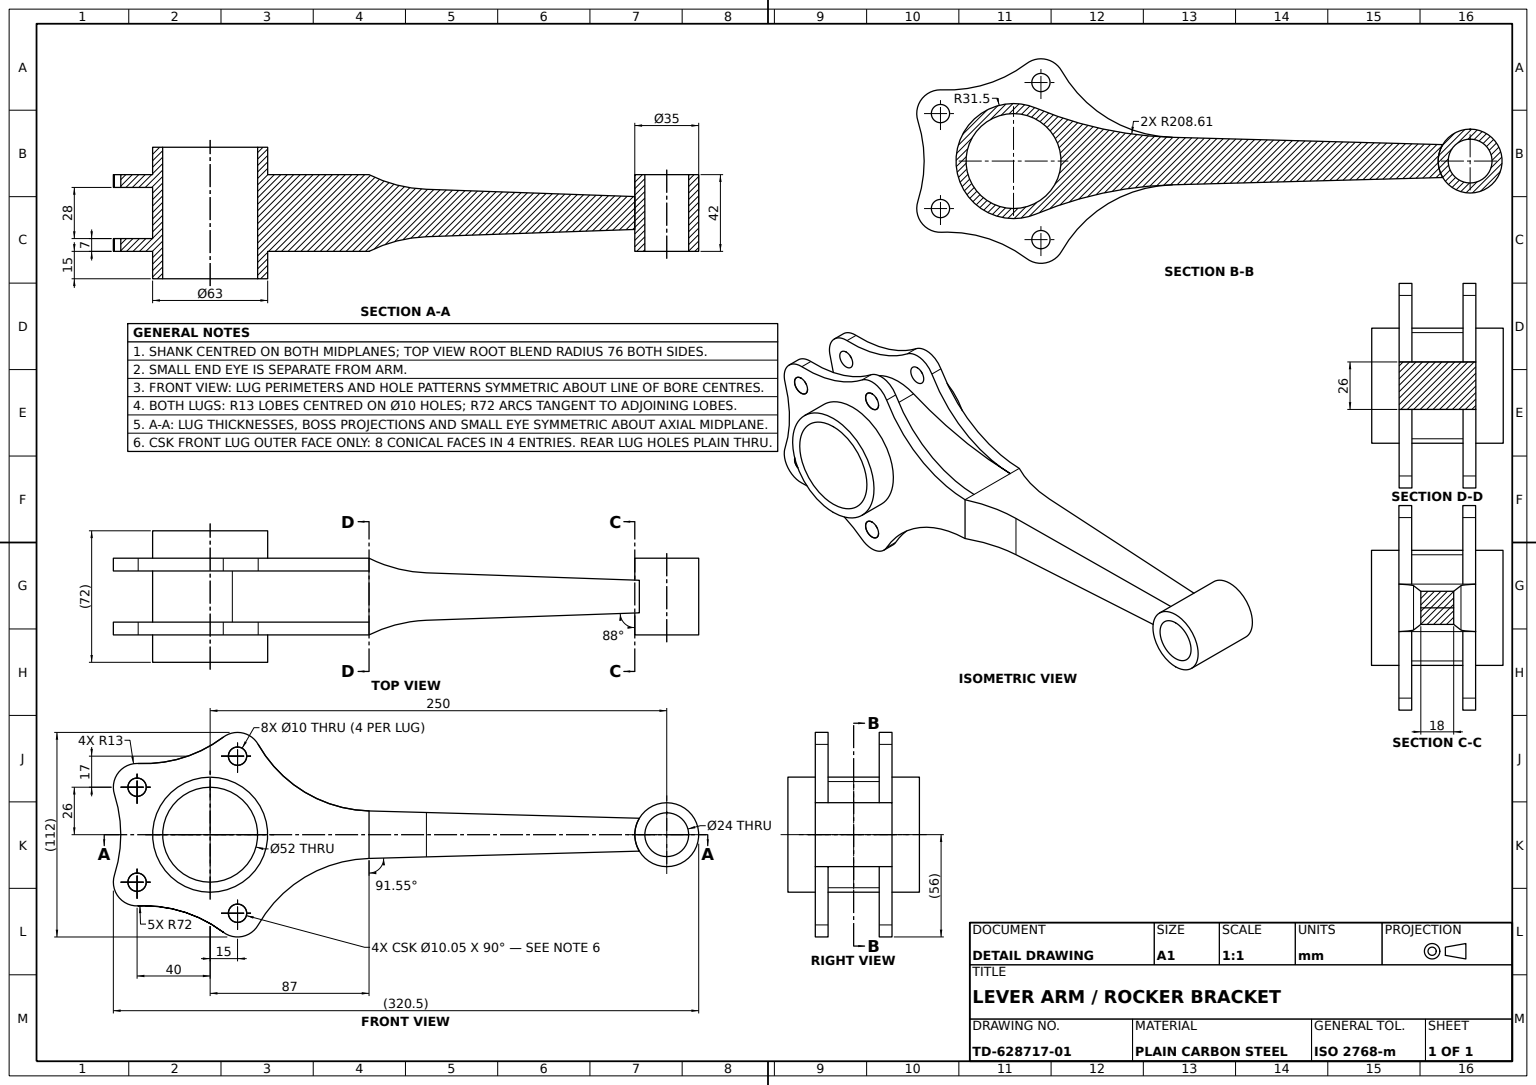
from build123d import *

# Parameters (mm, degrees)
ROD_PROFILE_SKETCH_R       = 31.5
ROD_PROFILE_SKETCH_R_2     = 26
ROD_BODY_DEPTH             = 36
SKETCH2_7_R                = 31.5
BIG_END_BOSS_DEPTH         = 21
SKETCH2_8_R                = 17.5
SKETCH2_8_R_2              = 12
SMALL_END_BOSS_DEPTH       = 21
BIG_END_CUT_DEPTH          = 14
BOLT_HOLES_10_AT_2_COUNT   = 2
BOLT_HOLES_10_AT_2_PITCH   = 57.567351858
BOLT_HOLES_10_AT_3_COUNT   = 2
BOLT_HOLES_10_AT_3_PITCH   = 86
BOLT_HOLES_10_AT_4_COUNT   = 2
BOLT_HOLES_10_AT_4_PITCH   = 88.238313674
SHANK_TAPER_CUT_DEPTH      = 276.659663353
SHANK_TAPER_CUT_DEPTH_BACK = 276.659663353


with BuildPart() as part:
    # Rod Profile Sketch → Rod Body (new, symmetric)
    with BuildSketch(Plane(origin=(0, 0, 0), x_dir=(1, 0, 0), z_dir=(0, 1, 0))):
        with Locations(Location((0, 0, 0), (0, 0, 270))):
            Circle(ROD_PROFILE_SKETCH_R)
        with Locations(Location((0, 0, 0), (0, 0, 270))):
            Circle(ROD_PROFILE_SKETCH_R_2, mode=Mode.SUBTRACT)
    extrude(amount=ROD_BODY_DEPTH, both=True)

    # Sketch2_7 → Big End Boss (add, symmetric)
    with BuildSketch(Plane(origin=(0, 0, 0), x_dir=(1, 0, 0), z_dir=(0, 1, 0))):
        with BuildLine():
            Line((86.968573361, -13), (234.99166898, -9))
            ThreePointArc((234.99166898, -9), (232.5, 0), (234.99166898, 9))
            Line((234.99166898, 9), (86.968573361, 13))
            ThreePointArc((86.968573361, 13), (51.854086448, 23.24367301), (26.304418517, 49.419511039))
            ThreePointArc((26.304418517, 49.419511039), (17.6406075, 55.72899022), (7.181946677, 53.386435492))
            ThreePointArc((7.181946677, 53.386435492), (-14.855989459, 42.122318837), (-39.406288617, 38.986435492))
            ThreePointArc((-39.406288617, 38.986435492), (-50.326951915, 33.896458963), (-52.376901133, 22.023529412))
            ThreePointArc((-52.376901133, 22.023529412), (-48.925892025, 0), (-52.376901133, -22.023529412))
            ThreePointArc((-52.376901133, -22.023529412), (-50.326951915, -33.896458963), (-39.406288617, -38.986435492))
            ThreePointArc((-39.406288617, -38.986435492), (-14.855989459, -42.122318837), (7.181946677, -53.386435492))
            ThreePointArc((7.181946677, -53.386435492), (17.6406075, -55.72899022), (26.304418517, -49.419511039))
            ThreePointArc((26.304418517, -49.419511039), (51.854086448, -23.24367301), (86.968573361, -13))
        make_face()
        with Locations(Location((0, 0, 0), (0, 0, 270))):
            Circle(SKETCH2_7_R, mode=Mode.SUBTRACT)
    extrude(amount=BIG_END_BOSS_DEPTH, both=True)

    # Big End Cut Sketch → Big End Cut (cut, symmetric)
    with BuildSketch(Plane(origin=(0, 0, 0), x_dir=(1, 0, 0), z_dir=(0, 1, 0))):
        with BuildLine():
            ThreePointArc((26.304418517, -49.419511039), (51.854086448, -23.24367301), (86.968573361, -13))
            ThreePointArc((86.968573361, -13), (48.815835223, -17.5713072), (12.14882026, -29.062968986))
            ThreePointArc((12.14882026, -29.062968986), (-31.5, 0), (12.14882026, 29.062968986))
            ThreePointArc((12.14882026, 29.062968986), (48.815835223, 17.5713072), (86.968573361, 13))
            ThreePointArc((86.968573361, 13), (51.854086448, 23.24367301), (26.304418517, 49.419511039))
            ThreePointArc((26.304418517, 49.419511039), (17.6406075, 55.72899022), (7.181946677, 53.386435492))
            ThreePointArc((7.181946677, 53.386435492), (-14.855989459, 42.122318837), (-39.406288617, 38.986435492))
            ThreePointArc((-39.406288617, 38.986435492), (-50.326951915, 33.896458963), (-52.376901133, 22.023529412))
            ThreePointArc((-52.376901133, 22.023529412), (-48.925892025, 0), (-52.376901133, -22.023529412))
            ThreePointArc((-52.376901133, -22.023529412), (-50.326951915, -33.896458963), (-39.406288617, -38.986435492))
            ThreePointArc((-39.406288617, -38.986435492), (-14.855989459, -42.122318837), (7.181946677, -53.386435492))
            ThreePointArc((7.181946677, -53.386435492), (17.6406075, -55.72899022), (26.304418517, -49.419511039))
        make_face()
    extrude(amount=BIG_END_CUT_DEPTH, both=True, mode=Mode.SUBTRACT)

    # Sketch9 → Bolt Holes _10 (revolve, cut)
    with BuildSketch(Plane(origin=(15, 21, -43), x_dir=(0, 0, 1), z_dir=(1, 0, 0))):
        Polygon((0, 0), (0, 57), (5, 57), (5, 0.025), (5.025, 0), align=None)
    bolt_holes_10 = revolve(axis=Axis((15, 27.35, -43), (0, -1, 0)), mode=Mode.SUBTRACT)

    # Bolt Holes _10 at 2: Bolt Holes _10 ×2
    with Locations(*[Vector(-0.9554026409829016, 0, 0.29530627084926053) * (i * BOLT_HOLES_10_AT_2_PITCH) for i in range(1, BOLT_HOLES_10_AT_2_COUNT)]):
        add(bolt_holes_10, mode=Mode.SUBTRACT)

    # Bolt Holes _10 at 3: Bolt Holes _10 ×2
    with Locations(*[(0, 0, i * BOLT_HOLES_10_AT_3_PITCH) for i in range(1, BOLT_HOLES_10_AT_3_COUNT)]):
        add(bolt_holes_10, mode=Mode.SUBTRACT)

    # Bolt Holes _10 at 4: Bolt Holes _10 ×2
    with Locations(*[Vector(-0.623312002576454, 0, 0.7819732395959151) * (i * BOLT_HOLES_10_AT_4_PITCH) for i in range(1, BOLT_HOLES_10_AT_4_COUNT)]):
        add(bolt_holes_10, mode=Mode.SUBTRACT)

    # Shank Taper Sketch → Shank Taper Cut (cut, two sides: drawn at the far end of the back side and taken through both)
    with BuildSketch(Plane.XY.offset(-SHANK_TAPER_CUT_DEPTH_BACK)):
        with BuildLine():
            Line((232.499010748, 9), (118.413371717, 12.983958303))
            ThreePointArc((118.413371717, 12.983958303), (102.27427636, 15.297447008), (87, 21))
            Line((87, 21), (232.499010748, 21))
            Line((232.499010748, 21), (250.081428832, 21))
            Line((250.081428832, 21), (250.081428832, 8.386008431))
            Line((250.081428832, 8.386008431), (232.499010748, 9))
        make_face()
        with BuildLine():
            Line((232.499010748, -21), (250.081428832, -21))
            Line((250.081428832, -21), (250.081428832, -8.386008431))
            Line((250.081428832, -8.386008431), (232.499010748, -9))
            Line((232.499010748, -9), (118.413371717, -12.983958303))
            ThreePointArc((118.413371717, -12.983958303), (102.27427636, -15.297447008), (87, -21))
            Line((87, -21), (232.499010748, -21))
        make_face()
    extrude(amount=SHANK_TAPER_CUT_DEPTH + SHANK_TAPER_CUT_DEPTH_BACK, mode=Mode.SUBTRACT)


with BuildPart() as body_2:
    # Sketch2_8 → Small End Boss (new, symmetric)
    with BuildSketch(Plane(origin=(0, 0, 0), x_dir=(1, 0, 0), z_dir=(0, 1, 0))):
        with Locations(Location((250, 0, 0), (0, 0, 90))):
            Circle(SKETCH2_8_R)
        with Locations(Location((250, 0, 0), (0, 0, 90))):
            Circle(SKETCH2_8_R_2, mode=Mode.SUBTRACT)
    extrude(amount=SMALL_END_BOSS_DEPTH, both=True)


solid = Compound([part.part, body_2.part])
